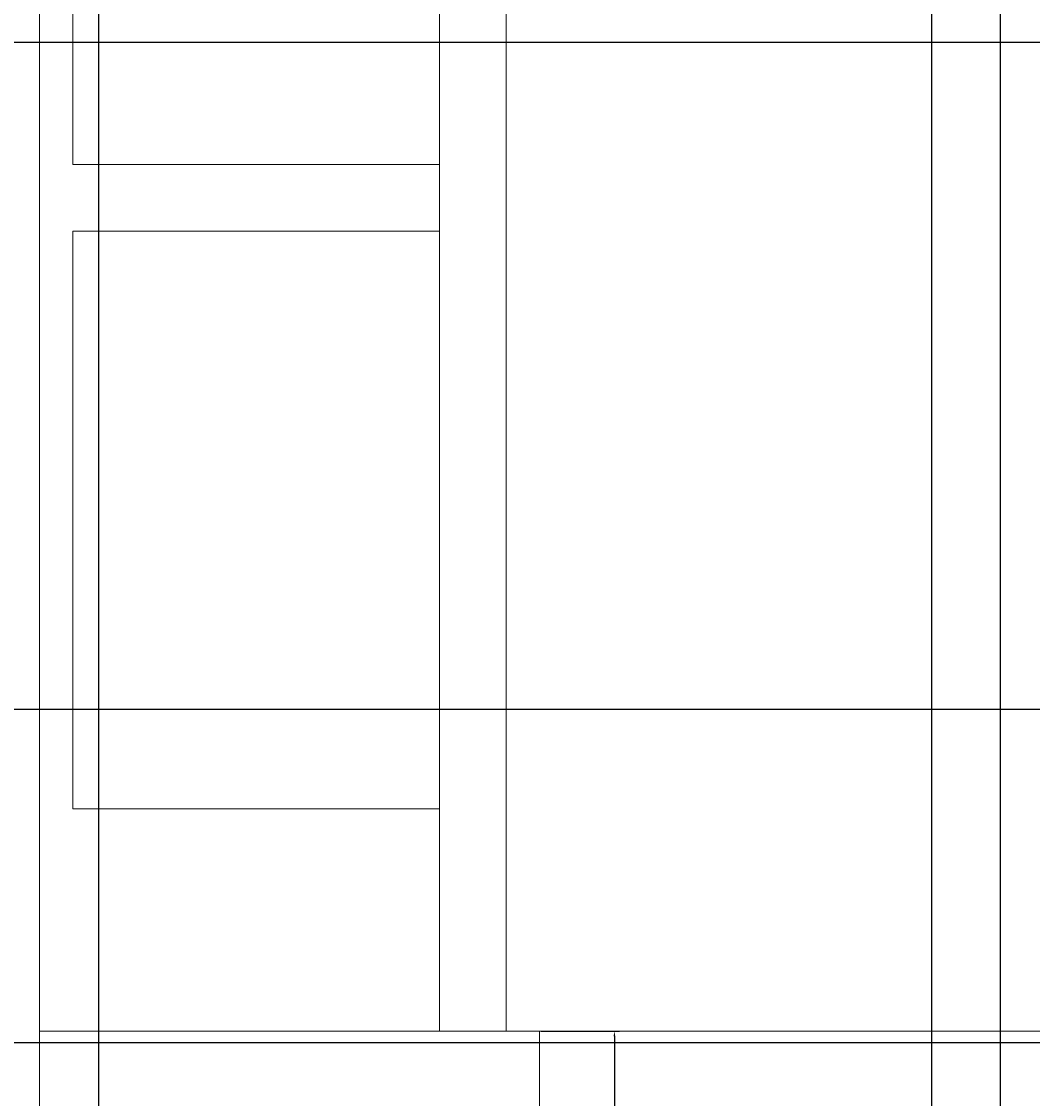
# Model space of a CAD drawing. Units: inches. Extents: x 2231 to 2461, y 2045 to 2455.
# Tile 70 of 95: x 2260 to 2296, y 2333 to 2372. Entities that reach past the tile are written whole.
import ezdxf

# ---------------------------------------------------------------- set-up
doc = ezdxf.new("R2010")
doc.units = ezdxf.units.IN
doc.layers.add('A-ANNO-DIMS', color=2, linetype='Continuous', lineweight=18)
doc.layers.add('A-FURN', color=9, linetype='Continuous', lineweight=18)
doc.styles.get("Standard").update_dxf_attribs({"font": 'arial.ttf'})
doc.dimstyles.get("Standard").update_dxf_attribs({"dimtxt": 0.18, "dimasz": 0.18, "dimexe": 0.18, "dimexo": 0.0625, "dimgap": 0.09, "dimtad": 0, "dimtih": 1, "dimtoh": 1, "dimdec": 4, "dimzin": 0, "dimdsep": 46, "dimtxsty": 'Standard', "dimcen": 0.09, "dimadec": 0, "dimazin": 0, "dimtfac": 1, "dimtdec": 4, "dimtofl": 0, "dimtmove": 0, "dimatfit": 3, "dimfxl": 1, "dimtolj": 1, "dimtzin": 0, "dimarcsym": 0})

# ---------------------------------------------------------------- blocks, each defined once
blk = doc.blocks.new('Bed - Queen')
for p, q in [((0, -80.00003), (0, 0)), ((0, 0), (59.99999, 0)), ((7.99999, -1.2), (28.79998, -1.2)), ((7.99999, -14.4), (7.99999, -1.2)), ((28.79998, -1.2), (28.79998, -14.4)), ((31.19999, -1.2), (51.99999, -1.2)), ((31.19999, -14.4), (31.19999, -1.2)), ((0, -14.4), (44.8, -14.4)), ((44.8, -16.8), (0, -16.8))]:
    blk.add_line(p, q)
blk = doc.blocks.new('NIGHTSTAND-18IN')
blk.add_lwpolyline([(0, 0), (18, 0), (18, 18), (0, 18)], close=True)
blk = doc.blocks.new('*D18')
at = {"layer": 'A-ANNO-DIMS', "color": 0, "lineweight": -2, "transparency": 16777216}
for p, q in [((2278.251, 2335.253), (2281.068, 2335.253)), ((2280.888, 2335.073), (2280.888, 2326.435)), ((2280.888, 2317.433), (2280.888, 2326.071)), ((2278.251, 2317.253), (2281.068, 2317.253))]:
    blk.add_line(p, q, dxfattribs=at)
at = {"layer": 'A-ANNO-DIMS', "color": 0, "transparency": 16777216}
for points in [[(2280.858, 2335.073), (2280.918, 2335.073), (2280.888, 2335.253)], [(2280.858, 2317.433), (2280.918, 2317.433), (2280.888, 2317.253)]]:
    blk.add_solid(points, dxfattribs=at)
at = {"layer": 'Defpoints', "color": 0, "transparency": 16777216}
for p in [(2278.188, 2335.253), (2280.888, 2335.253), (2278.188, 2317.253)]:
    blk.add_point(p, dxfattribs=at)
at = {"layer": 'A-ANNO-DIMS', "color": 0, "transparency": 16777216, "insert": (2280.888, 2326.253), "char_height": 0.18, "attachment_point": 5}
blk.add_mtext('\\A1;18 TYP.', dxfattribs=at)
blk = doc.blocks.new('*D47')
at = {"layer": 'A-ANNO-DIMS', "color": 0, "lineweight": -2, "transparency": 16777216}
for p, q in [((2258.794, 2182.895), (2258.794, 2454.645)), ((2258.974, 2454.465), (2276.575, 2454.465)), ((2294.614, 2454.465), (2277.012, 2454.465)), ((2294.794, 2182.895), (2294.794, 2454.645))]:
    blk.add_line(p, q, dxfattribs=at)
at = {"layer": 'A-ANNO-DIMS', "color": 0, "transparency": 16777216}
for points in [[(2258.974, 2454.495), (2258.974, 2454.435), (2258.794, 2454.465)], [(2294.614, 2454.495), (2294.614, 2454.435), (2294.794, 2454.465)]]:
    blk.add_solid(points, dxfattribs=at)
at = {"layer": 'Defpoints', "color": 0, "transparency": 16777216}
for p in [(2294.794, 2454.465), (2258.794, 2182.833), (2294.794, 2182.833)]:
    blk.add_point(p, dxfattribs=at)
at = {"layer": 'A-ANNO-DIMS', "color": 0, "transparency": 16777216, "insert": (2276.794, 2454.465), "char_height": 0.18, "attachment_point": 5}
blk.add_mtext('\\A1;36', dxfattribs=at)
blk = doc.blocks.new('*D53')
at = {"layer": 'A-ANNO-DIMS', "color": 0, "lineweight": -2, "transparency": 16777216}
for p, q in [((2372.731, 2346.833), (2230.981, 2346.833)), ((2231.161, 2346.653), (2231.161, 2341.013)), ((2231.161, 2335.013), (2231.161, 2340.652)), ((2372.731, 2334.833), (2230.981, 2334.833))]:
    blk.add_line(p, q, dxfattribs=at)
at = {"layer": 'A-ANNO-DIMS', "color": 0, "transparency": 16777216}
for points in [[(2231.131, 2346.653), (2231.191, 2346.653), (2231.161, 2346.833)], [(2231.131, 2335.013), (2231.191, 2335.013), (2231.161, 2334.833)]]:
    blk.add_solid(points, dxfattribs=at)
at = {"layer": 'Defpoints', "color": 0, "transparency": 16777216}
for p in [(2231.161, 2346.833), (2372.794, 2346.833), (2372.794, 2334.833)]:
    blk.add_point(p, dxfattribs=at)
at = {"layer": 'A-ANNO-DIMS', "color": 0, "transparency": 16777216, "insert": (2231.161, 2340.833), "char_height": 0.18, "attachment_point": 5}
blk.add_mtext('\\A1;12', dxfattribs=at)
blk = doc.blocks.new('*D54')
at = {"layer": 'A-ANNO-DIMS', "color": 0, "lineweight": -2, "transparency": 16777216}
for p, q in [((2372.731, 2370.833), (2230.981, 2370.833)), ((2231.161, 2370.653), (2231.161, 2359.013)), ((2231.161, 2347.013), (2231.161, 2358.652)), ((2372.731, 2346.833), (2230.981, 2346.833))]:
    blk.add_line(p, q, dxfattribs=at)
at = {"layer": 'A-ANNO-DIMS', "color": 0, "transparency": 16777216}
for points in [[(2231.131, 2370.653), (2231.191, 2370.653), (2231.161, 2370.833)], [(2231.131, 2347.013), (2231.191, 2347.013), (2231.161, 2346.833)]]:
    blk.add_solid(points, dxfattribs=at)
at = {"layer": 'Defpoints', "color": 0, "transparency": 16777216}
for p in [(2231.161, 2370.833), (2372.794, 2370.833), (2372.794, 2346.833)]:
    blk.add_point(p, dxfattribs=at)
at = {"layer": 'A-ANNO-DIMS', "color": 0, "transparency": 16777216, "insert": (2231.161, 2358.833), "char_height": 0.18, "attachment_point": 5}
blk.add_mtext('\\A1;24', dxfattribs=at)
blk = doc.blocks.new('*D62')
at = {"layer": 'A-ANNO-DIMS', "color": 0, "lineweight": -2, "transparency": 16777216}
for p, q in [((2262.321, 2255.176), (2262.321, 2454.645)), ((2262.501, 2454.465), (2277.102, 2454.465)), ((2292.141, 2454.465), (2277.539, 2454.465)), ((2292.321, 2253.176), (2292.321, 2454.645))]:
    blk.add_line(p, q, dxfattribs=at)
at = {"layer": 'A-ANNO-DIMS', "color": 0, "transparency": 16777216}
for points in [[(2262.501, 2454.495), (2262.501, 2454.435), (2262.321, 2454.465)], [(2292.141, 2454.495), (2292.141, 2454.435), (2292.321, 2454.465)]]:
    blk.add_solid(points, dxfattribs=at)
at = {"layer": 'Defpoints', "color": 0, "transparency": 16777216}
for p in [(2292.321, 2454.465), (2262.321, 2255.114), (2292.321, 2253.114)]:
    blk.add_point(p, dxfattribs=at)
at = {"layer": 'A-ANNO-DIMS', "color": 0, "transparency": 16777216, "insert": (2277.321, 2454.465), "char_height": 0.18, "attachment_point": 5}
blk.add_mtext('\\A1;30', dxfattribs=at)

msp = doc.modelspace()

# ---------------------------------------------------------------- block references
at = {"layer": 'A-FURN', "rotation": 90}
msp.add_blockref('Bed - Queen', (2260.1881, 2335.2534), dxfattribs=at)
at = {"layer": 'A-FURN'}
msp.add_blockref('NIGHTSTAND-18IN', (2260.188, 2317.253), dxfattribs=at)

# ---------------------------------------------------------------- dimensions: what is measured, and where the dimension line sits
at = {"layer": 'A-ANNO-DIMS'}
for base, p1, p2, picture, middle in [((2294.7935, 2454.4653), (2258.7935, 2182.8328), (2294.7935, 2182.8328), '*D47', (2276.7935, 2454.4653)), ((2292.3207, 2454.4653), (2262.3207, 2255.1137), (2292.3207, 2253.1137), '*D62', (2277.3207, 2454.4653))]:
    dim = msp.add_linear_dim(base=base, p1=p1, p2=p2, dimstyle='Standard', override={"dimdec": 0, "dimlfac": 1, "dimrnd": 0, "dimzin": 0, "dimdsep": 46, "dimlunit": 2}, dxfattribs=at)
    dim.commit()
    dim.dimension.update_dxf_attribs({"geometry": picture, "text_midpoint": middle})
for base, p1, p2, picture, middle in [((2231.161, 2370.8328), (2372.7935, 2346.8328), (2372.7935, 2370.8328), '*D54', (2231.161, 2358.8328)), ((2231.161, 2346.8328), (2372.7935, 2334.8328), (2372.7935, 2346.8328), '*D53', (2231.161, 2340.8328))]:
    dim = msp.add_linear_dim(base=base, p1=p1, p2=p2, angle=90, dimstyle='Standard', override={"dimdec": 0, "dimlfac": 1, "dimrnd": 0, "dimzin": 0, "dimdsep": 46, "dimlunit": 2}, dxfattribs=at)
    dim.commit()
    dim.dimension.update_dxf_attribs({"geometry": picture, "text_midpoint": middle})
dim = msp.add_linear_dim(base=(2280.8881, 2335.2534), p1=(2278.1881, 2317.2534), p2=(2278.1881, 2335.2534), angle=90, text='<> TYP.', dimstyle='Standard', override={"dimdec": 0, "dimlfac": 1, "dimrnd": 0, "dimzin": 0, "dimdsep": 46, "dimlunit": 2}, dxfattribs=at)
dim.commit()
dim.dimension.update_dxf_attribs({"geometry": '*D18', "text_midpoint": (2280.8881, 2326.2534)})

doc.saveas('drawing.dxf')
